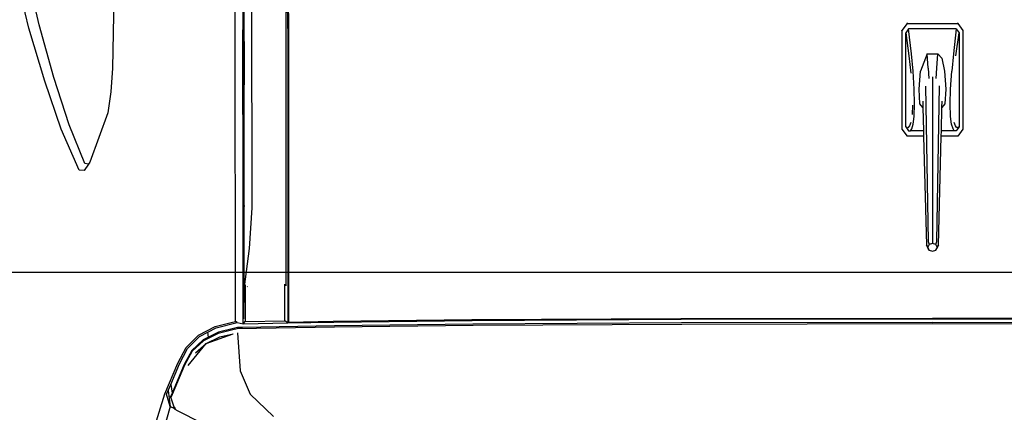
# Model space of a CAD drawing. Units: inches. Extents: x 1319 to 2030, y 219 to 1069.
# Tile 6 of 28: x 1434 to 1464, y 380 to 392. Entities that reach past the tile are written whole.
import ezdxf

# ---------------------------------------------------------------- set-up
doc = ezdxf.new("R2010")
doc.units = ezdxf.units.IN
doc.header["$MEASUREMENT"] = 0
doc.layers.get('0').update_dxf_attribs({"color": 12})
doc.layers.add('A-ANNO-DIMS', color=2, linetype='Continuous', lineweight=18)
doc.layers.add('C-PRKG-VEHC', color=8, linetype='Continuous', lineweight=13)
doc.layers.add('Edges', color=250, linetype='Continuous')
doc.styles.get("Standard").update_dxf_attribs({"font": 'arial.ttf'})
doc.dimstyles.get("Standard").update_dxf_attribs({"dimtxt": 7, "dimasz": 0.18, "dimexe": 0.18, "dimexo": 0.0625, "dimgap": 0.09, "dimtad": 0, "dimtih": 1, "dimtoh": 1, "dimzin": 0, "dimdsep": 46, "dimlunit": 3, "dimtxsty": 'Standard', "dimcen": 0.09, "dimadec": 0, "dimazin": 0, "dimtfac": 1, "dimtofl": 0, "dimtmove": 0, "dimatfit": 3, "dimfxl": 1, "dimtolj": 1, "dimtzin": 0, "dimarcsym": 0})

# ---------------------------------------------------------------- blocks, each defined once
blk = doc.blocks.new('Nissan Qashqai pl')
at = {"layer": 'Edges'}
for p, q in [((11.05474, 11.92208), (11.05507, 12.12031)), ((11.05537, 11.92208), (11.05571, 12.1202)), ((11.0586, 12.11975), (11.05827, 11.92208)), ((11.05972, 12.11965), (11.05938, 11.92208)), ((10.8228, 11.94208), (10.82239, 11.94208)), ((10.8228, 11.94208), (10.82834, 11.94608)), ((10.8228, 11.90208), (10.8228, 11.94208)), ((10.82696, 11.94083), (10.83007, 11.94308)), ((10.82794, 11.94608), (10.82834, 11.94608)), ((10.82834, 11.94608), (10.90603, 11.94608)), ((10.84833, 11.9406), (10.83007, 11.94308)), ((10.83007, 11.94308), (10.9043, 11.94308)), ((10.9043, 11.94308), (10.90741, 11.94083)), ((10.9043, 11.94308), (10.90503, 11.94137)), ((10.90603, 11.94608), (10.91157, 11.94208)), ((10.91157, 11.94208), (10.91157, 11.92904)), ((10.82696, 11.94083), (10.82696, 11.90333)), ((10.82696, 11.94083), (10.84666, 11.93861)), ((10.84666, 11.93861), (10.86027, 11.93735)), ((10.8746, 11.93634), (10.86027, 11.93735)), ((10.88611, 11.93611), (10.8746, 11.93634)), ((10.89593, 11.93645), (10.88611, 11.93611)), ((10.90215, 11.93722), (10.89593, 11.93645)), ((10.90348, 11.94026), (10.90076, 11.93914)), ((10.90565, 11.93837), (10.90215, 11.93722)), ((10.90503, 11.94137), (10.90348, 11.94026)), ((10.90744, 11.9393), (10.90565, 11.93837)), ((10.90741, 11.94083), (10.90744, 11.9393)), ((10.90744, 11.9393), (10.90744, 11.92915)), ((10.84666, 11.92634), (10.85007, 11.92947)), ((10.85007, 11.92947), (10.86027, 11.93157)), ((10.86027, 11.93157), (10.8746, 11.93265)), ((10.99456, 11.92544), (10.87195, 11.92764)), ((10.8746, 11.93265), (10.88611, 11.93193)), ((10.889, 11.92962), (10.88395, 11.92975)), ((10.88611, 11.93193), (10.889, 11.92962)), ((10.90744, 11.92915), (10.889, 11.92962)), ((10.91157, 11.92904), (10.90744, 11.92915)), ((10.99731, 11.92683), (10.91157, 11.92904)), ((10.99731, 11.92683), (11.00007, 11.92544)), ((10.99903, 11.92575), (10.99731, 11.92683)), ((10.84666, 11.91782), (10.84666, 11.92634)), ((10.85787, 11.92547), (10.84666, 11.92634)), ((10.86624, 11.92503), (10.85787, 11.92547)), ((10.85787, 11.91869), (10.86624, 11.91913)), ((10.86474, 11.92208), (10.99603, 11.92208)), ((10.99691, 11.92468), (10.99456, 11.92544)), ((10.99456, 11.91872), (10.99691, 11.91949)), ((10.99691, 11.92468), (10.99603, 11.92208)), ((10.99603, 11.92208), (10.99691, 11.91949)), ((10.99903, 11.92575), (10.99691, 11.92468)), ((10.99691, 11.91949), (10.99903, 11.91841)), ((11.00116, 11.92468), (10.99903, 11.92575)), ((10.99963, 11.91871), (11.00116, 11.91949)), ((11.00116, 11.92468), (11.00007, 11.92544)), ((11.00116, 11.91949), (11.00007, 11.91872)), ((11.00204, 11.92208), (11.00116, 11.92468)), ((11.00116, 11.91949), (11.00204, 11.92208)), ((11.05507, 11.72385), (11.05474, 11.92208)), ((11.05571, 11.72396), (11.05537, 11.92208)), ((11.05827, 11.92208), (11.0586, 11.72441)), ((11.05938, 11.92208), (11.05972, 11.72451)), ((10.85787, 11.91869), (10.84666, 11.91782)), ((10.84666, 11.91782), (10.86027, 11.91259)), ((10.8746, 11.91151), (10.86027, 11.91259)), ((10.87225, 11.91653), (10.99456, 11.91872)), ((10.88611, 11.91223), (10.8746, 11.91151)), ((10.88395, 11.91441), (10.889, 11.91454)), ((10.889, 11.91454), (10.88611, 11.91223)), ((10.889, 11.91454), (10.90744, 11.91502)), ((10.90744, 11.91502), (10.91157, 11.91512)), ((10.90744, 11.91502), (10.90744, 11.90486)), ((10.91157, 11.91512), (10.99731, 11.91733)), ((10.91157, 11.91512), (10.91157, 11.90208)), ((11.00007, 11.91872), (10.99731, 11.91733)), ((10.99731, 11.91733), (10.99903, 11.91841)), ((10.99903, 11.91841), (10.99963, 11.91871)), ((11.00007, 11.91872), (10.99963, 11.91871)), ((10.84666, 11.90555), (10.82696, 11.90333)), ((10.82696, 11.90333), (10.83007, 11.90108)), ((10.83007, 11.90108), (10.84833, 11.90356)), ((10.86027, 11.90681), (10.84666, 11.90555)), ((10.84833, 11.90356), (10.86193, 11.905)), ((10.8746, 11.90782), (10.86027, 11.90681)), ((10.88611, 11.90805), (10.8746, 11.90782)), ((10.89593, 11.90771), (10.88611, 11.90805)), ((10.88709, 11.90634), (10.89442, 11.90601)), ((10.90215, 11.90694), (10.89593, 11.90771)), ((10.90076, 11.90502), (10.90348, 11.9039)), ((10.90565, 11.90579), (10.90215, 11.90694)), ((10.90348, 11.9039), (10.90503, 11.90279)), ((10.9043, 11.90108), (10.90741, 11.90333)), ((10.90744, 11.90486), (10.90565, 11.90579)), ((10.90741, 11.90333), (10.90744, 11.90486)), ((10.90741, 11.90333), (10.90741, 11.90484)), ((10.82239, 11.90208), (10.8228, 11.90208)), ((10.8228, 11.90208), (10.82834, 11.89808)), ((10.82834, 11.89808), (10.82794, 11.89808)), ((10.82834, 11.89808), (10.90603, 11.89808)), ((10.9043, 11.90108), (10.83007, 11.90108)), ((10.90503, 11.90279), (10.9043, 11.90108)), ((10.90603, 11.89808), (10.91157, 11.90208)), ((11.05596, 11.55904), (11.05507, 11.72385)), ((11.0566, 11.5593), (11.05571, 11.72396)), ((11.0586, 11.72441), (11.05947, 11.55994)), ((11.05972, 11.72451), (11.06059, 11.56009)), ((11.05722, 11.44991), (11.05596, 11.55904)), ((11.05785, 11.45038), (11.0566, 11.5593)), ((11.05947, 11.55994), (11.06074, 11.45082)), ((11.06059, 11.56009), (11.06182, 11.4509)), ((11.05789, 11.4146), (11.05722, 11.44991)), ((11.05854, 11.41419), (11.05785, 11.45038)), ((11.06074, 11.45082), (11.06214, 11.37845)), ((11.06182, 11.4509), (11.06324, 11.37414)), ((10.79328, 11.41432), (10.82704, 11.4145)), ((10.82704, 11.4145), (11.05789, 11.4146)), ((11.05854, 11.41419), (11.05789, 11.4146)), ((10.7493, 11.41253), (11.02943, 11.41262)), ((10.82673, 11.41408), (10.79328, 11.4139)), ((10.82673, 11.41408), (11.05854, 11.41419)), ((11.02945, 11.41183), (11.02814, 11.41183)), ((11.02944, 11.41252), (11.02943, 11.41262)), ((11.05683, 11.41184), (11.02945, 11.41183)), ((11.02945, 11.41162), (11.02945, 11.41183)), ((11.05854, 11.41419), (11.05683, 11.41184)), ((11.05743, 11.38044), (11.05683, 11.41184)), ((11.05921, 11.37886), (11.05854, 11.41419)), ((11.11477, 11.38434), (11.1323, 11.40268)), ((10.75022, 11.38554), (10.96805, 11.38566)), ((10.96805, 11.38566), (10.99996, 11.38365)), ((10.99996, 11.38365), (11.03007, 11.37965)), ((11.09618, 11.37663), (11.11477, 11.38434)), ((10.69998, 11.37799), (10.82786, 11.37874)), ((10.78083, 11.37927), (10.8711, 11.37956)), ((10.94306, 11.3796), (10.82786, 11.37874)), ((10.82786, 11.37874), (11.05524, 11.37886)), ((10.96142, 11.37881), (10.82786, 11.37874)), ((10.89604, 11.37957), (10.8711, 11.37956)), ((10.90974, 11.3796), (10.89604, 11.37957)), ((10.94306, 11.3796), (10.90974, 11.3796)), ((10.94785, 11.37963), (10.94306, 11.3796)), ((10.9491, 11.37964), (10.94785, 11.37963)), ((10.96679, 11.37961), (10.9491, 11.37964)), ((10.96142, 11.37881), (10.96679, 11.37961)), ((10.97113, 11.37881), (10.96142, 11.37881)), ((10.96679, 11.37961), (10.96696, 11.37964)), ((10.97653, 11.37962), (10.96696, 11.37964)), ((10.97653, 11.37962), (10.97113, 11.37881)), ((10.97664, 11.37882), (10.97113, 11.37881)), ((10.98248, 11.37964), (10.97653, 11.37962)), ((10.97653, 11.37962), (10.97664, 11.37882)), ((11.05921, 11.37886), (10.97664, 11.37882)), ((11.03007, 11.37965), (10.98248, 11.37964)), ((11.02869, 11.38043), (11.03005, 11.38043)), ((11.03005, 11.38025), (11.02923, 11.38024)), ((11.03002, 11.38217), (11.03001, 11.38239)), ((11.03005, 11.38043), (11.05544, 11.38044)), ((11.05544, 11.38044), (11.03005, 11.38025)), ((11.03005, 11.38025), (11.03005, 11.38043)), ((11.03007, 11.37965), (11.03005, 11.38025)), ((11.05544, 11.38044), (11.05743, 11.38044)), ((11.05921, 11.37886), (11.05743, 11.38044)), ((11.05822, 11.37418), (11.05921, 11.37886)), ((11.06214, 11.37845), (11.06222, 11.37449)), ((11.06624, 11.37435), (11.09618, 11.37663)), ((10.82794, 11.37265), (10.7004, 11.37196)), ((11.05437, 11.37279), (10.82794, 11.37265)), ((11.05754, 11.37277), (11.05437, 11.37279)), ((11.05822, 11.37418), (11.05754, 11.37277)), ((11.05807, 11.37037), (11.05754, 11.37277)), ((11.06139, 11.35691), (11.05807, 11.37037)), ((11.06236, 11.3576), (11.05822, 11.37418)), ((11.06222, 11.37449), (11.06303, 11.37135)), ((11.06303, 11.37135), (11.06594, 11.3594)), ((11.06324, 11.37414), (11.06408, 11.37085)), ((11.06408, 11.37085), (11.06692, 11.35921)), ((11.06961, 11.36056), (11.0671, 11.37109)), ((11.07472, 11.34981), (11.0671, 11.37109)), ((11.07472, 11.34981), (11.06961, 11.36056)), ((11.06818, 11.34377), (11.06139, 11.35691)), ((11.06584, 11.35092), (11.06236, 11.3576)), ((11.06594, 11.3594), (11.06978, 11.35164)), ((11.06692, 11.35921), (11.0727, 11.34754)), ((11.06978, 11.35164), (11.06584, 11.35092)), ((11.06918, 11.34452), (11.06584, 11.35092)), ((11.06978, 11.35164), (11.07183, 11.3475)), ((11.07183, 11.3475), (11.08018, 11.33842)), ((11.0727, 11.34754), (11.0809, 11.33858)), ((11.08206, 11.34125), (11.07472, 11.34981)), ((11.092, 11.33548), (11.07472, 11.34981)), ((11.12767, 11.32749), (11.13692, 11.34555)), ((11.07787, 11.3339), (11.06818, 11.34377)), ((11.07866, 11.33492), (11.06918, 11.34452)), ((11.08018, 11.33842), (11.09121, 11.33249)), ((11.0809, 11.33858), (11.09174, 11.33271)), ((11.09022, 11.32753), (11.07787, 11.3339)), ((11.09081, 11.32882), (11.07866, 11.33492)), ((11.09121, 11.33249), (11.1138, 11.3229)), ((11.09174, 11.33271), (11.11486, 11.323)), ((11.11439, 11.31711), (11.09022, 11.32753)), ((11.10704, 11.32181), (11.09081, 11.32882)), ((11.10704, 11.32181), (11.1138, 11.3229)), ((11.11164, 11.31982), (11.10704, 11.32181)), ((11.11164, 11.31982), (11.1244, 11.32146)), ((11.1138, 11.3229), (11.11393, 11.32284)), ((11.11393, 11.32284), (11.1164, 11.32172)), ((11.1244, 11.32146), (11.11467, 11.31851)), ((11.11486, 11.323), (11.1172, 11.32196)), ((11.1164, 11.32172), (11.1172, 11.32196)), ((11.11744, 11.32189), (11.1164, 11.32172)), ((11.1172, 11.32196), (11.11744, 11.32189)), ((11.11744, 11.32189), (11.11997, 11.32267)), ((11.11997, 11.32267), (11.12459, 11.32429)), ((11.12604, 11.32481), (11.1244, 11.32146)), ((11.1244, 11.32146), (11.12591, 11.32476)), ((11.1244, 11.32146), (11.16836, 11.30873)), ((11.12459, 11.32429), (11.12591, 11.32476)), ((11.12466, 11.32442), (11.12595, 11.32486)), ((11.12478, 11.32467), (11.12595, 11.32486)), ((11.12595, 11.32486), (11.1251, 11.3253)), ((11.12591, 11.32476), (11.12595, 11.32486)), ((11.12591, 11.32476), (11.12604, 11.32481)), ((11.12595, 11.32486), (11.12626, 11.32554)), ((11.12595, 11.32486), (11.12607, 11.32488)), ((11.12604, 11.32481), (11.12645, 11.32495)), ((11.12607, 11.32488), (11.12604, 11.32481)), ((11.12631, 11.32537), (11.12607, 11.32488)), ((11.12607, 11.32488), (11.12645, 11.32495)), ((11.12645, 11.32495), (11.12767, 11.32749)), ((11.11467, 11.31851), (11.11164, 11.31982)), ((11.17021, 11.29978), (11.11439, 11.31711)), ((10.77686, 11.27742), (10.85804, 11.27587)), ((10.85804, 11.27587), (10.87661, 11.27449)), ((10.87661, 11.27449), (10.89318, 11.27219)), ((10.89318, 11.27219), (10.932, 11.25799)), ((10.93299, 11.25409), (10.90264, 11.24169)), ((10.932, 11.25799), (10.93345, 11.25704)), ((10.93345, 11.25704), (10.93299, 11.25409)), ((10.93345, 11.25704), (10.93862, 11.25365)), ((10.93862, 11.25365), (10.9384, 11.24966)), ((10.9384, 11.24966), (10.90591, 11.23547)), ((10.90264, 11.24169), (10.86528, 11.22973)), ((10.86528, 11.22973), (10.82385, 11.21811)), ((10.90591, 11.23547), (10.86821, 11.22258)), ((10.86821, 11.22258), (10.82645, 11.21003)), ((10.82385, 11.21811), (10.77536, 11.20713)), ((10.82645, 11.21003), (10.77763, 11.19817))]:
    blk.add_line(p, q, dxfattribs=at)
blk = doc.blocks.new('car')
blk.add_blockref('Nissan Qashqai pl', (-9.74328, -11.91512))
blk = doc.blocks.new('carr')
blk.add_blockref('car', (0.51244, -0.00696))
blk = doc.blocks.new('*D65')
at = {"layer": 'A-ANNO-DIMS', "color": 0, "lineweight": -2, "transparency": 16777216}
for p, q in [((1648.280254, 472.227245), (1329.112754, 472.227245)), ((1329.292754, 472.047245), (1329.292754, 431.817245)), ((1329.292754, 384.407245), (1329.292754, 424.637245)), ((1648.280254, 384.227245), (1329.112754, 384.227245))]:
    blk.add_line(p, q, dxfattribs=at)
at = {"layer": 'A-ANNO-DIMS', "color": 0, "transparency": 16777216}
for points in [[(1329.262754, 472.047245), (1329.322754, 472.047245), (1329.292754, 472.227245)], [(1329.262754, 384.407245), (1329.322754, 384.407245), (1329.292754, 384.227245)]]:
    blk.add_solid(points, dxfattribs=at)
at = {"layer": 'Defpoints', "color": 0, "transparency": 16777216}
for p in [(1329.292754, 472.227245), (1648.342754, 472.227245), (1648.342754, 384.227245)]:
    blk.add_point(p, dxfattribs=at)
at = {"layer": 'A-ANNO-DIMS', "color": 0, "transparency": 16777216, "insert": (1329.292754, 428.227245), "char_height": 7, "attachment_point": 5}
blk.add_mtext('\\A1;7\'-4"', dxfattribs=at)

msp = doc.modelspace()

# ---------------------------------------------------------------- block references
at = {"layer": 'C-PRKG-VEHC', "xscale": 39.37007874015748, "yscale": 39.37007874015748, "zscale": 39.37007874015748, "rotation": 270}
msp.add_blockref('carr', (1462.179, 454.621), dxfattribs=at)

# ---------------------------------------------------------------- dimensions: what is measured, and where the dimension line sits
at = {"layer": 'A-ANNO-DIMS'}
dim = msp.add_linear_dim(base=(1329.293, 472.227), p1=(1648.343, 384.227), p2=(1648.343, 472.227), angle=90, dimstyle='Standard', override={"dimdec": 1, "dimlfac": 1, "dimrnd": 0, "dimzin": 1, "dimdsep": 46, "dimlunit": 4, "dimfrac": 2}, dxfattribs=at)
dim.commit()
dim.dimension.update_dxf_attribs({"geometry": '*D65', "text_midpoint": (1329.293, 428.227)})

doc.saveas('drawing.dxf')
